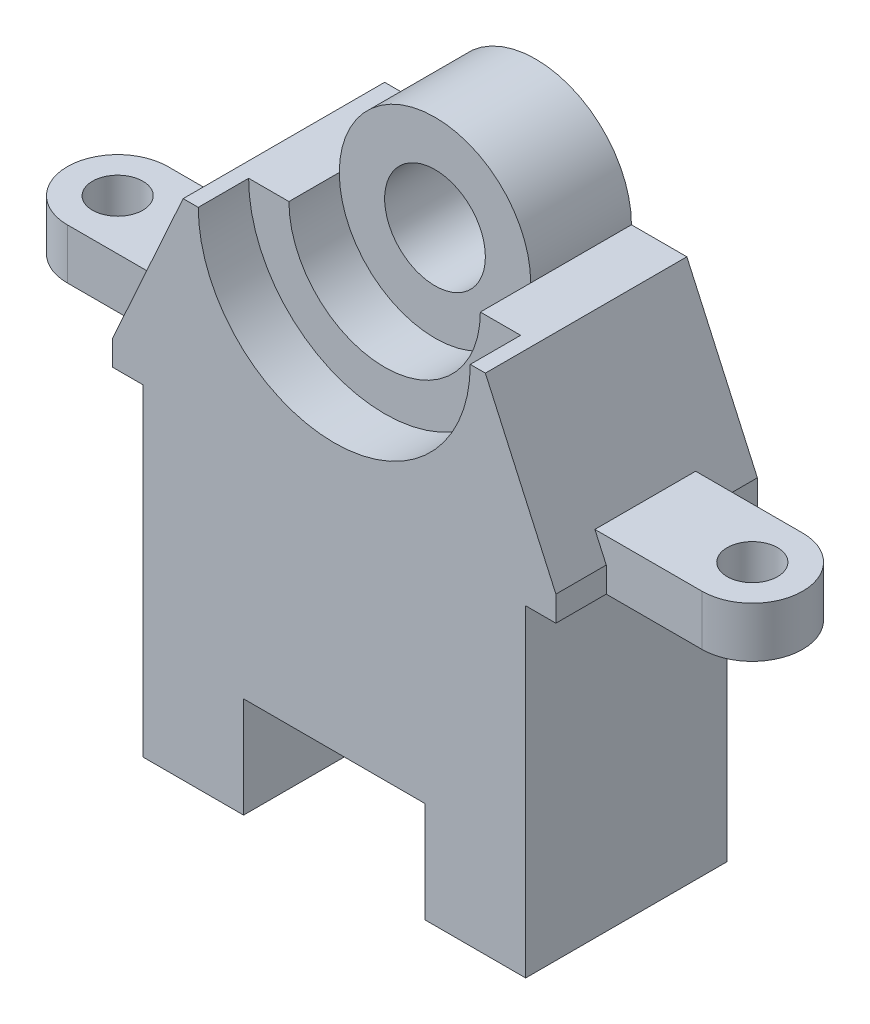
ISO-10303-21;
HEADER;
FILE_DESCRIPTION(('STEP AP214'),'2;1');
FILE_NAME('part.step','',(''),(''),'','','');
FILE_SCHEMA(('AUTOMOTIVE_DESIGN { 1 0 10303 214 1 1 1 1 }'));
ENDSEC;
DATA;
#1=APPLICATION_CONTEXT('core data for automotive mechanical design processes');
#2=APPLICATION_PROTOCOL_DEFINITION('international standard','automotive_design',2000,#1);
#3=PRODUCT_CONTEXT('',#1,'mechanical');
#4=PRODUCT('Part','Part','',(#3));
#5=PRODUCT_RELATED_PRODUCT_CATEGORY('part','',(#4));
#6=PRODUCT_DEFINITION_FORMATION('','',#4);
#7=PRODUCT_DEFINITION_CONTEXT('part definition',#1,'design');
#8=PRODUCT_DEFINITION('design','',#6,#7);
#9=PRODUCT_DEFINITION_SHAPE('','',#8);
#10=(LENGTH_UNIT() NAMED_UNIT(*) SI_UNIT(.MILLI.,.METRE.));
#11=(NAMED_UNIT(*) PLANE_ANGLE_UNIT() SI_UNIT($,.RADIAN.));
#12=(NAMED_UNIT(*) SI_UNIT($,.STERADIAN.) SOLID_ANGLE_UNIT());
#13=UNCERTAINTY_MEASURE_WITH_UNIT(LENGTH_MEASURE(1.E-05),#10,'distance_accuracy_value','');
#14=(GEOMETRIC_REPRESENTATION_CONTEXT(3) GLOBAL_UNCERTAINTY_ASSIGNED_CONTEXT((#13)) GLOBAL_UNIT_ASSIGNED_CONTEXT((#10,
#11,#12)) REPRESENTATION_CONTEXT('',''));
#15=CARTESIAN_POINT('',(0.,0.,0.));
#16=DIRECTION('',(0.,0.,1.));
#17=DIRECTION('',(1.,0.,0.));
#18=AXIS2_PLACEMENT_3D('',#15,#16,#17);
#19=CARTESIAN_POINT('',(44.,37.,20.));
#20=DIRECTION('',(-1.,0.,0.));
#21=DIRECTION('',(0.,0.,1.));
#22=AXIS2_PLACEMENT_3D('',#19,#20,#21);
#23=PLANE('',#22);
#24=DIRECTION('',(0.,1.,0.));
#25=VECTOR('',#24,1.);
#26=CARTESIAN_POINT('',(44.,37.,-10.));
#27=LINE('',#26,#25);
#28=CARTESIAN_POINT('',(44.,32.,-10.));
#29=VERTEX_POINT('',#28);
#30=CARTESIAN_POINT('',(44.,37.,-10.));
#31=VERTEX_POINT('',#30);
#32=EDGE_CURVE('E58',#29,#31,#27,.T.);
#33=ORIENTED_EDGE('',*,*,#32,.F.);
#34=DIRECTION('',(0.,0.,-1.));
#35=VECTOR('',#34,1.);
#36=CARTESIAN_POINT('',(44.,32.,20.));
#37=LINE('',#36,#35);
#38=CARTESIAN_POINT('',(44.,32.,-20.));
#39=VERTEX_POINT('',#38);
#40=EDGE_CURVE('E459',#29,#39,#37,.T.);
#41=ORIENTED_EDGE('',*,*,#40,.T.);
#42=DIRECTION('',(0.,1.,0.));
#43=VECTOR('',#42,1.);
#44=CARTESIAN_POINT('',(44.,37.,-20.));
#45=LINE('',#44,#43);
#46=CARTESIAN_POINT('',(44.,37.,-20.));
#47=VERTEX_POINT('',#46);
#48=EDGE_CURVE('E386',#39,#47,#45,.T.);
#49=ORIENTED_EDGE('',*,*,#48,.T.);
#50=DIRECTION('',(0.,0.,-1.));
#51=VECTOR('',#50,1.);
#52=CARTESIAN_POINT('',(44.,37.,20.));
#53=LINE('',#52,#51);
#54=EDGE_CURVE('E457',#31,#47,#53,.T.);
#55=ORIENTED_EDGE('',*,*,#54,.F.);
#56=EDGE_LOOP('',(#33,#41,#49,#55));
#57=FACE_BOUND('',#56,.T.);
#58=ADVANCED_FACE('F44',(#57),#23,.F.);
#59=DIRECTION('',(0.,-1.,0.));
#60=VECTOR('',#59,1.);
#61=CARTESIAN_POINT('',(44.,37.,10.));
#62=LINE('',#61,#60);
#63=CARTESIAN_POINT('',(44.,37.,10.));
#64=VERTEX_POINT('',#63);
#65=CARTESIAN_POINT('',(44.,32.,10.));
#66=VERTEX_POINT('',#65);
#67=EDGE_CURVE('E274',#64,#66,#62,.T.);
#68=ORIENTED_EDGE('',*,*,#67,.F.);
#69=CARTESIAN_POINT('',(44.,37.,20.));
#70=VERTEX_POINT('',#69);
#71=EDGE_CURVE('E460',#70,#64,#53,.T.);
#72=ORIENTED_EDGE('',*,*,#71,.F.);
#73=DIRECTION('',(0.,1.,0.));
#74=VECTOR('',#73,1.);
#75=CARTESIAN_POINT('',(44.,37.,20.));
#76=LINE('',#75,#74);
#77=CARTESIAN_POINT('',(44.,32.,20.));
#78=VERTEX_POINT('',#77);
#79=EDGE_CURVE('E357',#78,#70,#76,.T.);
#80=ORIENTED_EDGE('',*,*,#79,.F.);
#81=EDGE_CURVE('E69',#78,#66,#37,.T.);
#82=ORIENTED_EDGE('',*,*,#81,.T.);
#83=EDGE_LOOP('',(#68,#72,#80,#82));
#84=FACE_BOUND('',#83,.T.);
#85=ADVANCED_FACE('F476',(#84),#23,.F.);
#86=CARTESIAN_POINT('',(30.,68.,20.));
#87=DIRECTION('',(-0.911370599658675,-0.411586722426498,0.));
#88=DIRECTION('',(0.411586722426498,-0.911370599658675,0.));
#89=AXIS2_PLACEMENT_3D('',#86,#87,#88);
#90=PLANE('',#89);
#91=DIRECTION('',(-0.411586722426498,0.911370599658675,0.));
#92=VECTOR('',#91,1.);
#93=CARTESIAN_POINT('',(30.,68.,-10.));
#94=LINE('',#93,#92);
#95=CARTESIAN_POINT('',(41.741935483871,42.,-10.));
#96=VERTEX_POINT('',#95);
#97=EDGE_CURVE('E11',#31,#96,#94,.T.);
#98=ORIENTED_EDGE('',*,*,#97,.F.);
#99=ORIENTED_EDGE('',*,*,#54,.T.);
#100=DIRECTION('',(-0.411586722426498,0.911370599658675,0.));
#101=VECTOR('',#100,1.);
#102=CARTESIAN_POINT('',(30.,68.,-20.));
#103=LINE('',#102,#101);
#104=CARTESIAN_POINT('',(30.,68.,-20.));
#105=VERTEX_POINT('',#104);
#106=EDGE_CURVE('E394',#47,#105,#103,.T.);
#107=ORIENTED_EDGE('',*,*,#106,.T.);
#108=DIRECTION('',(0.,0.,-1.));
#109=VECTOR('',#108,1.);
#110=CARTESIAN_POINT('',(30.,68.,20.));
#111=LINE('',#110,#109);
#112=CARTESIAN_POINT('',(30.,68.,20.));
#113=VERTEX_POINT('',#112);
#114=EDGE_CURVE('E454',#113,#105,#111,.T.);
#115=ORIENTED_EDGE('',*,*,#114,.F.);
#116=DIRECTION('',(-0.411586722426498,0.911370599658675,0.));
#117=VECTOR('',#116,1.);
#118=CARTESIAN_POINT('',(30.,68.,20.));
#119=LINE('',#118,#117);
#120=EDGE_CURVE('E360',#70,#113,#119,.T.);
#121=ORIENTED_EDGE('',*,*,#120,.F.);
#122=ORIENTED_EDGE('',*,*,#71,.T.);
#123=DIRECTION('',(0.411586722426498,-0.911370599658675,0.));
#124=VECTOR('',#123,1.);
#125=CARTESIAN_POINT('',(30.,68.,10.));
#126=LINE('',#125,#124);
#127=CARTESIAN_POINT('',(41.741935483871,42.,10.));
#128=VERTEX_POINT('',#127);
#129=EDGE_CURVE('E472',#128,#64,#126,.T.);
#130=ORIENTED_EDGE('',*,*,#129,.F.);
#131=DIRECTION('',(0.,0.,1.));
#132=VECTOR('',#131,1.);
#133=CARTESIAN_POINT('',(41.741935483871,42.,20.));
#134=LINE('',#133,#132);
#135=EDGE_CURVE('E52',#96,#128,#134,.T.);
#136=ORIENTED_EDGE('',*,*,#135,.F.);
#137=EDGE_LOOP('',(#98,#99,#107,#115,#121,#122,#130,#136));
#138=FACE_BOUND('',#137,.T.);
#139=ADVANCED_FACE('F475',(#138),#90,.F.);
#140=CARTESIAN_POINT('',(-44.,32.,20.));
#141=DIRECTION('',(1.,0.,0.));
#142=DIRECTION('',(0.,0.,-1.));
#143=AXIS2_PLACEMENT_3D('',#140,#141,#142);
#144=PLANE('',#143);
#145=DIRECTION('',(0.,0.,-1.));
#146=VECTOR('',#145,1.);
#147=CARTESIAN_POINT('',(-44.,37.,20.));
#148=LINE('',#147,#146);
#149=CARTESIAN_POINT('',(-44.,37.,20.));
#150=VERTEX_POINT('',#149);
#151=CARTESIAN_POINT('',(-44.,37.,10.));
#152=VERTEX_POINT('',#151);
#153=EDGE_CURVE('E449',#150,#152,#148,.T.);
#154=ORIENTED_EDGE('',*,*,#153,.T.);
#155=DIRECTION('',(0.,-1.,0.));
#156=VECTOR('',#155,1.);
#157=CARTESIAN_POINT('',(-44.,32.,10.));
#158=LINE('',#157,#156);
#159=CARTESIAN_POINT('',(-44.,32.,10.));
#160=VERTEX_POINT('',#159);
#161=EDGE_CURVE('E315',#152,#160,#158,.T.);
#162=ORIENTED_EDGE('',*,*,#161,.T.);
#163=DIRECTION('',(0.,0.,-1.));
#164=VECTOR('',#163,1.);
#165=CARTESIAN_POINT('',(-44.,32.,20.));
#166=LINE('',#165,#164);
#167=CARTESIAN_POINT('',(-44.,32.,20.));
#168=VERTEX_POINT('',#167);
#169=EDGE_CURVE('E444',#168,#160,#166,.T.);
#170=ORIENTED_EDGE('',*,*,#169,.F.);
#171=DIRECTION('',(0.,-1.,0.));
#172=VECTOR('',#171,1.);
#173=CARTESIAN_POINT('',(-44.,32.,20.));
#174=LINE('',#173,#172);
#175=EDGE_CURVE('E366',#150,#168,#174,.T.);
#176=ORIENTED_EDGE('',*,*,#175,.F.);
#177=EDGE_LOOP('',(#154,#162,#170,#176));
#178=FACE_BOUND('',#177,.T.);
#179=ADVANCED_FACE('F482',(#178),#144,.F.);
#180=CARTESIAN_POINT('',(-30.,68.,20.));
#181=DIRECTION('',(0.,-1.,0.));
#182=DIRECTION('',(0.,0.,-1.));
#183=AXIS2_PLACEMENT_3D('',#180,#181,#182);
#184=PLANE('',#183);
#185=DIRECTION('',(-1.,0.,0.));
#186=VECTOR('',#185,1.);
#187=CARTESIAN_POINT('',(-30.,68.,-20.));
#188=LINE('',#187,#186);
#189=CARTESIAN_POINT('',(19.,68.,-20.));
#190=VERTEX_POINT('',#189);
#191=EDGE_CURVE('E391',#105,#190,#188,.T.);
#192=ORIENTED_EDGE('',*,*,#191,.T.);
#193=DIRECTION('',(0.,0.,1.));
#194=VECTOR('',#193,1.);
#195=CARTESIAN_POINT('',(19.,68.,-73.7401153701776));
#196=LINE('',#195,#194);
#197=CARTESIAN_POINT('',(19.,68.,0.));
#198=VERTEX_POINT('',#197);
#199=EDGE_CURVE('E335',#190,#198,#196,.T.);
#200=ORIENTED_EDGE('',*,*,#199,.T.);
#201=DIRECTION('',(0.,0.,1.));
#202=VECTOR('',#201,1.);
#203=CARTESIAN_POINT('',(19.,68.,0.));
#204=LINE('',#203,#202);
#205=CARTESIAN_POINT('',(19.,68.,10.));
#206=VERTEX_POINT('',#205);
#207=EDGE_CURVE('E341',#198,#206,#204,.T.);
#208=ORIENTED_EDGE('',*,*,#207,.T.);
#209=DIRECTION('',(-1.,0.,0.));
#210=VECTOR('',#209,1.);
#211=CARTESIAN_POINT('',(-30.,68.,10.));
#212=LINE('',#211,#210);
#213=CARTESIAN_POINT('',(27.,68.,10.));
#214=VERTEX_POINT('',#213);
#215=EDGE_CURVE('E461',#214,#206,#212,.T.);
#216=ORIENTED_EDGE('',*,*,#215,.F.);
#217=DIRECTION('',(0.,0.,1.));
#218=VECTOR('',#217,1.);
#219=CARTESIAN_POINT('',(27.,68.,10.));
#220=LINE('',#219,#218);
#221=CARTESIAN_POINT('',(27.,68.,20.));
#222=VERTEX_POINT('',#221);
#223=EDGE_CURVE('E348',#214,#222,#220,.T.);
#224=ORIENTED_EDGE('',*,*,#223,.T.);
#225=DIRECTION('',(-1.,0.,0.));
#226=VECTOR('',#225,1.);
#227=CARTESIAN_POINT('',(-30.,68.,20.));
#228=LINE('',#227,#226);
#229=EDGE_CURVE('E361',#113,#222,#228,.T.);
#230=ORIENTED_EDGE('',*,*,#229,.F.);
#231=ORIENTED_EDGE('',*,*,#114,.T.);
#232=EDGE_LOOP('',(#192,#200,#208,#216,#224,#230,#231));
#233=FACE_BOUND('',#232,.T.);
#234=ADVANCED_FACE('F495',(#233),#184,.F.);
#235=CARTESIAN_POINT('',(44.,32.,20.));
#236=DIRECTION('',(0.,1.,0.));
#237=DIRECTION('',(0.,0.,1.));
#238=AXIS2_PLACEMENT_3D('',#235,#236,#237);
#239=PLANE('',#238);
#240=DIRECTION('',(0.,0.,-1.));
#241=VECTOR('',#240,1.);
#242=CARTESIAN_POINT('',(38.,32.,20.));
#243=LINE('',#242,#241);
#244=CARTESIAN_POINT('',(38.,32.,20.));
#245=VERTEX_POINT('',#244);
#246=CARTESIAN_POINT('',(38.,32.,-20.));
#247=VERTEX_POINT('',#246);
#248=EDGE_CURVE('E387',#245,#247,#243,.T.);
#249=ORIENTED_EDGE('',*,*,#248,.T.);
#250=DIRECTION('',(1.,0.,0.));
#251=VECTOR('',#250,1.);
#252=CARTESIAN_POINT('',(44.,32.,-20.));
#253=LINE('',#252,#251);
#254=EDGE_CURVE('E352',#247,#39,#253,.T.);
#255=ORIENTED_EDGE('',*,*,#254,.T.);
#256=ORIENTED_EDGE('',*,*,#40,.F.);
#257=DIRECTION('',(-1.,0.,0.));
#258=VECTOR('',#257,1.);
#259=CARTESIAN_POINT('',(63.,32.,-10.));
#260=LINE('',#259,#258);
#261=CARTESIAN_POINT('',(63.,32.,-10.));
#262=VERTEX_POINT('',#261);
#263=EDGE_CURVE('E265',#262,#29,#260,.T.);
#264=ORIENTED_EDGE('',*,*,#263,.F.);
#265=CARTESIAN_POINT('',(63.,32.,0.));
#266=DIRECTION('',(0.,1.,0.));
#267=DIRECTION('',(0.,0.,-1.));
#268=AXIS2_PLACEMENT_3D('',#265,#266,#267);
#269=CIRCLE('',#268,10.);
#270=CARTESIAN_POINT('',(63.,32.,10.));
#271=VERTEX_POINT('',#270);
#272=EDGE_CURVE('E271',#271,#262,#269,.T.);
#273=ORIENTED_EDGE('',*,*,#272,.F.);
#274=DIRECTION('',(1.,0.,0.));
#275=VECTOR('',#274,1.);
#276=CARTESIAN_POINT('',(44.,32.,10.));
#277=LINE('',#276,#275);
#278=EDGE_CURVE('E255',#66,#271,#277,.T.);
#279=ORIENTED_EDGE('',*,*,#278,.F.);
#280=ORIENTED_EDGE('',*,*,#81,.F.);
#281=DIRECTION('',(1.,0.,0.));
#282=VECTOR('',#281,1.);
#283=CARTESIAN_POINT('',(44.,32.,20.));
#284=LINE('',#283,#282);
#285=EDGE_CURVE('E355',#245,#78,#284,.T.);
#286=ORIENTED_EDGE('',*,*,#285,.F.);
#287=EDGE_LOOP('',(#249,#255,#256,#264,#273,#279,#280,#286));
#288=FACE_BOUND('',#287,.T.);
#289=CARTESIAN_POINT('',(63.,32.,0.));
#290=DIRECTION('',(0.,1.,0.));
#291=DIRECTION('',(0.,0.,-1.));
#292=AXIS2_PLACEMENT_3D('',#289,#290,#291);
#293=CIRCLE('',#292,5.);
#294=CARTESIAN_POINT('',(63.,32.,-5.));
#295=VERTEX_POINT('',#294);
#296=EDGE_CURVE('E270',#295,#295,#293,.T.);
#297=ORIENTED_EDGE('',*,*,#296,.T.);
#298=EDGE_LOOP('',(#297));
#299=FACE_BOUND('',#298,.T.);
#300=ADVANCED_FACE('F50',(#288,#299),#239,.F.);
#301=DIRECTION('',(0.,0.,1.));
#302=VECTOR('',#301,1.);
#303=CARTESIAN_POINT('',(-19.,68.,0.));
#304=LINE('',#303,#302);
#305=CARTESIAN_POINT('',(-19.,68.,10.));
#306=VERTEX_POINT('',#305);
#307=CARTESIAN_POINT('',(-19.,68.,0.));
#308=VERTEX_POINT('',#307);
#309=EDGE_CURVE('E337',#306,#308,#304,.F.);
#310=ORIENTED_EDGE('',*,*,#309,.T.);
#311=DIRECTION('',(0.,0.,1.));
#312=VECTOR('',#311,1.);
#313=CARTESIAN_POINT('',(-19.,68.,-73.7401153701776));
#314=LINE('',#313,#312);
#315=CARTESIAN_POINT('',(-19.,68.,-20.));
#316=VERTEX_POINT('',#315);
#317=EDGE_CURVE('E328',#308,#316,#314,.F.);
#318=ORIENTED_EDGE('',*,*,#317,.T.);
#319=CARTESIAN_POINT('',(-30.,68.,-20.));
#320=VERTEX_POINT('',#319);
#321=EDGE_CURVE('E395',#316,#320,#188,.T.);
#322=ORIENTED_EDGE('',*,*,#321,.T.);
#323=DIRECTION('',(0.,0.,-1.));
#324=VECTOR('',#323,1.);
#325=CARTESIAN_POINT('',(-30.,68.,20.));
#326=LINE('',#325,#324);
#327=CARTESIAN_POINT('',(-30.,68.,20.));
#328=VERTEX_POINT('',#327);
#329=EDGE_CURVE('E446',#328,#320,#326,.T.);
#330=ORIENTED_EDGE('',*,*,#329,.F.);
#331=CARTESIAN_POINT('',(-27.,68.,20.));
#332=VERTEX_POINT('',#331);
#333=EDGE_CURVE('E362',#332,#328,#228,.T.);
#334=ORIENTED_EDGE('',*,*,#333,.F.);
#335=DIRECTION('',(0.,0.,1.));
#336=VECTOR('',#335,1.);
#337=CARTESIAN_POINT('',(-27.,68.,10.));
#338=LINE('',#337,#336);
#339=CARTESIAN_POINT('',(-27.,68.,10.));
#340=VERTEX_POINT('',#339);
#341=EDGE_CURVE('E350',#332,#340,#338,.F.);
#342=ORIENTED_EDGE('',*,*,#341,.T.);
#343=EDGE_CURVE('E465',#306,#340,#212,.T.);
#344=ORIENTED_EDGE('',*,*,#343,.F.);
#345=EDGE_LOOP('',(#310,#318,#322,#330,#334,#342,#344));
#346=FACE_BOUND('',#345,.T.);
#347=ADVANCED_FACE('F490',(#346),#184,.F.);
#348=CARTESIAN_POINT('',(-44.,37.,20.));
#349=DIRECTION('',(0.911370599658675,-0.411586722426498,0.));
#350=DIRECTION('',(0.411586722426498,0.911370599658675,0.));
#351=AXIS2_PLACEMENT_3D('',#348,#349,#350);
#352=PLANE('',#351);
#353=DIRECTION('',(0.,0.,-1.));
#354=VECTOR('',#353,1.);
#355=CARTESIAN_POINT('',(-41.741935483871,42.,20.));
#356=LINE('',#355,#354);
#357=CARTESIAN_POINT('',(-41.741935483871,42.,10.));
#358=VERTEX_POINT('',#357);
#359=CARTESIAN_POINT('',(-41.741935483871,42.,-10.));
#360=VERTEX_POINT('',#359);
#361=EDGE_CURVE('E470',#358,#360,#356,.T.);
#362=ORIENTED_EDGE('',*,*,#361,.F.);
#363=DIRECTION('',(-0.411586722426498,-0.911370599658675,0.));
#364=VECTOR('',#363,1.);
#365=CARTESIAN_POINT('',(-44.,37.,10.));
#366=LINE('',#365,#364);
#367=EDGE_CURVE('E312',#358,#152,#366,.T.);
#368=ORIENTED_EDGE('',*,*,#367,.T.);
#369=ORIENTED_EDGE('',*,*,#153,.F.);
#370=DIRECTION('',(-0.411586722426498,-0.911370599658675,0.));
#371=VECTOR('',#370,1.);
#372=CARTESIAN_POINT('',(-44.,37.,20.));
#373=LINE('',#372,#371);
#374=EDGE_CURVE('E368',#328,#150,#373,.T.);
#375=ORIENTED_EDGE('',*,*,#374,.F.);
#376=ORIENTED_EDGE('',*,*,#329,.T.);
#377=DIRECTION('',(-0.411586722426498,-0.911370599658675,0.));
#378=VECTOR('',#377,1.);
#379=CARTESIAN_POINT('',(-44.,37.,-20.));
#380=LINE('',#379,#378);
#381=CARTESIAN_POINT('',(-44.,37.,-20.));
#382=VERTEX_POINT('',#381);
#383=EDGE_CURVE('E399',#320,#382,#380,.T.);
#384=ORIENTED_EDGE('',*,*,#383,.T.);
#385=CARTESIAN_POINT('',(-44.,37.,-10.));
#386=VERTEX_POINT('',#385);
#387=EDGE_CURVE('E448',#386,#382,#148,.T.);
#388=ORIENTED_EDGE('',*,*,#387,.F.);
#389=DIRECTION('',(0.411586722426498,0.911370599658675,0.));
#390=VECTOR('',#389,1.);
#391=CARTESIAN_POINT('',(-44.,37.,-10.));
#392=LINE('',#391,#390);
#393=EDGE_CURVE('E310',#386,#360,#392,.T.);
#394=ORIENTED_EDGE('',*,*,#393,.T.);
#395=EDGE_LOOP('',(#362,#368,#369,#375,#376,#384,#388,#394));
#396=FACE_BOUND('',#395,.T.);
#397=ADVANCED_FACE('F489',(#396),#352,.F.);
#398=CARTESIAN_POINT('',(-44.,32.,-10.));
#399=VERTEX_POINT('',#398);
#400=CARTESIAN_POINT('',(-44.,32.,-20.));
#401=VERTEX_POINT('',#400);
#402=EDGE_CURVE('E445',#399,#401,#166,.T.);
#403=ORIENTED_EDGE('',*,*,#402,.F.);
#404=DIRECTION('',(0.,1.,0.));
#405=VECTOR('',#404,1.);
#406=CARTESIAN_POINT('',(-44.,32.,-10.));
#407=LINE('',#406,#405);
#408=EDGE_CURVE('E303',#399,#386,#407,.T.);
#409=ORIENTED_EDGE('',*,*,#408,.T.);
#410=ORIENTED_EDGE('',*,*,#387,.T.);
#411=DIRECTION('',(0.,-1.,0.));
#412=VECTOR('',#411,1.);
#413=CARTESIAN_POINT('',(-44.,32.,-20.));
#414=LINE('',#413,#412);
#415=EDGE_CURVE('E402',#382,#401,#414,.T.);
#416=ORIENTED_EDGE('',*,*,#415,.T.);
#417=EDGE_LOOP('',(#403,#409,#410,#416));
#418=FACE_BOUND('',#417,.T.);
#419=ADVANCED_FACE('F494',(#418),#144,.F.);
#420=CARTESIAN_POINT('',(-38.,32.,20.));
#421=DIRECTION('',(0.,1.,0.));
#422=DIRECTION('',(0.,0.,1.));
#423=AXIS2_PLACEMENT_3D('',#420,#421,#422);
#424=PLANE('',#423);
#425=DIRECTION('',(1.,0.,0.));
#426=VECTOR('',#425,1.);
#427=CARTESIAN_POINT('',(-38.,32.,-20.));
#428=LINE('',#427,#426);
#429=CARTESIAN_POINT('',(-38.,32.,-20.));
#430=VERTEX_POINT('',#429);
#431=EDGE_CURVE('E404',#401,#430,#428,.T.);
#432=ORIENTED_EDGE('',*,*,#431,.T.);
#433=DIRECTION('',(0.,0.,-1.));
#434=VECTOR('',#433,1.);
#435=CARTESIAN_POINT('',(-38.,32.,20.));
#436=LINE('',#435,#434);
#437=CARTESIAN_POINT('',(-38.,32.,20.));
#438=VERTEX_POINT('',#437);
#439=EDGE_CURVE('E439',#438,#430,#436,.T.);
#440=ORIENTED_EDGE('',*,*,#439,.F.);
#441=DIRECTION('',(1.,0.,0.));
#442=VECTOR('',#441,1.);
#443=CARTESIAN_POINT('',(-38.,32.,20.));
#444=LINE('',#443,#442);
#445=EDGE_CURVE('E367',#168,#438,#444,.T.);
#446=ORIENTED_EDGE('',*,*,#445,.F.);
#447=ORIENTED_EDGE('',*,*,#169,.T.);
#448=DIRECTION('',(-1.,0.,0.));
#449=VECTOR('',#448,1.);
#450=CARTESIAN_POINT('',(-63.,32.,10.));
#451=LINE('',#450,#449);
#452=CARTESIAN_POINT('',(-63.,32.,10.));
#453=VERTEX_POINT('',#452);
#454=EDGE_CURVE('E290',#160,#453,#451,.T.);
#455=ORIENTED_EDGE('',*,*,#454,.T.);
#456=CARTESIAN_POINT('',(-63.,32.,0.));
#457=DIRECTION('',(0.,-1.,0.));
#458=DIRECTION('',(0.,0.,-1.));
#459=AXIS2_PLACEMENT_3D('',#456,#457,#458);
#460=CIRCLE('',#459,10.);
#461=CARTESIAN_POINT('',(-63.,32.,-10.));
#462=VERTEX_POINT('',#461);
#463=EDGE_CURVE('E282',#453,#462,#460,.T.);
#464=ORIENTED_EDGE('',*,*,#463,.T.);
#465=DIRECTION('',(1.,0.,0.));
#466=VECTOR('',#465,1.);
#467=CARTESIAN_POINT('',(-38.,32.,-10.));
#468=LINE('',#467,#466);
#469=EDGE_CURVE('E297',#462,#399,#468,.T.);
#470=ORIENTED_EDGE('',*,*,#469,.T.);
#471=ORIENTED_EDGE('',*,*,#402,.T.);
#472=EDGE_LOOP('',(#432,#440,#446,#447,#455,#464,#470,#471));
#473=FACE_BOUND('',#472,.T.);
#474=CARTESIAN_POINT('',(-63.,32.,0.));
#475=DIRECTION('',(0.,-1.,0.));
#476=DIRECTION('',(0.,0.,-1.));
#477=AXIS2_PLACEMENT_3D('',#474,#475,#476);
#478=CIRCLE('',#477,5.);
#479=CARTESIAN_POINT('',(-63.,32.,-5.));
#480=VERTEX_POINT('',#479);
#481=EDGE_CURVE('E276',#480,#480,#478,.T.);
#482=ORIENTED_EDGE('',*,*,#481,.F.);
#483=EDGE_LOOP('',(#482));
#484=FACE_BOUND('',#483,.T.);
#485=ADVANCED_FACE('F496',(#473,#484),#424,.F.);
#486=CARTESIAN_POINT('',(-38.,-32.,20.));
#487=DIRECTION('',(1.,0.,0.));
#488=DIRECTION('',(0.,0.,-1.));
#489=AXIS2_PLACEMENT_3D('',#486,#487,#488);
#490=PLANE('',#489);
#491=DIRECTION('',(0.,-1.,0.));
#492=VECTOR('',#491,1.);
#493=CARTESIAN_POINT('',(-38.,-32.,-20.));
#494=LINE('',#493,#492);
#495=CARTESIAN_POINT('',(-38.,-32.,-20.));
#496=VERTEX_POINT('',#495);
#497=EDGE_CURVE('E409',#430,#496,#494,.T.);
#498=ORIENTED_EDGE('',*,*,#497,.T.);
#499=DIRECTION('',(0.,0.,-1.));
#500=VECTOR('',#499,1.);
#501=CARTESIAN_POINT('',(-38.,-32.,20.));
#502=LINE('',#501,#500);
#503=CARTESIAN_POINT('',(-38.,-32.,20.));
#504=VERTEX_POINT('',#503);
#505=EDGE_CURVE('E440',#504,#496,#502,.T.);
#506=ORIENTED_EDGE('',*,*,#505,.F.);
#507=DIRECTION('',(0.,-1.,0.));
#508=VECTOR('',#507,1.);
#509=CARTESIAN_POINT('',(-38.,-32.,20.));
#510=LINE('',#509,#508);
#511=EDGE_CURVE('E375',#438,#504,#510,.T.);
#512=ORIENTED_EDGE('',*,*,#511,.F.);
#513=ORIENTED_EDGE('',*,*,#439,.T.);
#514=EDGE_LOOP('',(#498,#506,#512,#513));
#515=FACE_BOUND('',#514,.T.);
#516=ADVANCED_FACE('F502',(#515),#490,.F.);
#517=CARTESIAN_POINT('',(-38.,-32.,20.));
#518=DIRECTION('',(0.,1.,0.));
#519=DIRECTION('',(0.,0.,1.));
#520=AXIS2_PLACEMENT_3D('',#517,#518,#519);
#521=PLANE('',#520);
#522=DIRECTION('',(1.,0.,0.));
#523=VECTOR('',#522,1.);
#524=CARTESIAN_POINT('',(-38.,-32.,-20.));
#525=LINE('',#524,#523);
#526=CARTESIAN_POINT('',(-18.,-32.,-20.));
#527=VERTEX_POINT('',#526);
#528=EDGE_CURVE('E410',#496,#527,#525,.T.);
#529=ORIENTED_EDGE('',*,*,#528,.T.);
#530=DIRECTION('',(0.,0.,-1.));
#531=VECTOR('',#530,1.);
#532=CARTESIAN_POINT('',(-18.,-32.,20.));
#533=LINE('',#532,#531);
#534=CARTESIAN_POINT('',(-18.,-32.,20.));
#535=VERTEX_POINT('',#534);
#536=EDGE_CURVE('E432',#535,#527,#533,.T.);
#537=ORIENTED_EDGE('',*,*,#536,.F.);
#538=DIRECTION('',(1.,0.,0.));
#539=VECTOR('',#538,1.);
#540=CARTESIAN_POINT('',(-38.,-32.,20.));
#541=LINE('',#540,#539);
#542=EDGE_CURVE('E372',#504,#535,#541,.T.);
#543=ORIENTED_EDGE('',*,*,#542,.F.);
#544=ORIENTED_EDGE('',*,*,#505,.T.);
#545=EDGE_LOOP('',(#529,#537,#543,#544));
#546=FACE_BOUND('',#545,.T.);
#547=ADVANCED_FACE('F507',(#546),#521,.F.);
#548=CARTESIAN_POINT('',(-18.,-32.,20.));
#549=DIRECTION('',(-1.,0.,0.));
#550=DIRECTION('',(0.,0.,1.));
#551=AXIS2_PLACEMENT_3D('',#548,#549,#550);
#552=PLANE('',#551);
#553=DIRECTION('',(0.,1.,0.));
#554=VECTOR('',#553,1.);
#555=CARTESIAN_POINT('',(-18.,-32.,-20.));
#556=LINE('',#555,#554);
#557=CARTESIAN_POINT('',(-18.,-12.,-20.));
#558=VERTEX_POINT('',#557);
#559=EDGE_CURVE('E411',#527,#558,#556,.T.);
#560=ORIENTED_EDGE('',*,*,#559,.T.);
#561=DIRECTION('',(0.,0.,-1.));
#562=VECTOR('',#561,1.);
#563=CARTESIAN_POINT('',(-18.,-12.,20.));
#564=LINE('',#563,#562);
#565=CARTESIAN_POINT('',(-18.,-12.,20.));
#566=VERTEX_POINT('',#565);
#567=EDGE_CURVE('E431',#566,#558,#564,.T.);
#568=ORIENTED_EDGE('',*,*,#567,.F.);
#569=DIRECTION('',(0.,1.,0.));
#570=VECTOR('',#569,1.);
#571=CARTESIAN_POINT('',(-18.,-32.,20.));
#572=LINE('',#571,#570);
#573=EDGE_CURVE('E376',#535,#566,#572,.T.);
#574=ORIENTED_EDGE('',*,*,#573,.F.);
#575=ORIENTED_EDGE('',*,*,#536,.T.);
#576=EDGE_LOOP('',(#560,#568,#574,#575));
#577=FACE_BOUND('',#576,.T.);
#578=ADVANCED_FACE('F512',(#577),#552,.F.);
#579=CARTESIAN_POINT('',(-18.,-12.,20.));
#580=DIRECTION('',(0.,1.,0.));
#581=DIRECTION('',(0.,0.,1.));
#582=AXIS2_PLACEMENT_3D('',#579,#580,#581);
#583=PLANE('',#582);
#584=DIRECTION('',(1.,0.,0.));
#585=VECTOR('',#584,1.);
#586=CARTESIAN_POINT('',(-18.,-12.,-20.));
#587=LINE('',#586,#585);
#588=CARTESIAN_POINT('',(18.,-12.,-20.));
#589=VERTEX_POINT('',#588);
#590=EDGE_CURVE('E414',#558,#589,#587,.T.);
#591=ORIENTED_EDGE('',*,*,#590,.T.);
#592=DIRECTION('',(0.,0.,-1.));
#593=VECTOR('',#592,1.);
#594=CARTESIAN_POINT('',(18.,-12.,20.));
#595=LINE('',#594,#593);
#596=CARTESIAN_POINT('',(18.,-12.,20.));
#597=VERTEX_POINT('',#596);
#598=EDGE_CURVE('E428',#597,#589,#595,.T.);
#599=ORIENTED_EDGE('',*,*,#598,.F.);
#600=DIRECTION('',(1.,0.,0.));
#601=VECTOR('',#600,1.);
#602=CARTESIAN_POINT('',(-18.,-12.,20.));
#603=LINE('',#602,#601);
#604=EDGE_CURVE('E378',#566,#597,#603,.T.);
#605=ORIENTED_EDGE('',*,*,#604,.F.);
#606=ORIENTED_EDGE('',*,*,#567,.T.);
#607=EDGE_LOOP('',(#591,#599,#605,#606));
#608=FACE_BOUND('',#607,.T.);
#609=ADVANCED_FACE('F513',(#608),#583,.F.);
#610=CARTESIAN_POINT('',(18.,-32.,20.));
#611=DIRECTION('',(1.,0.,0.));
#612=DIRECTION('',(0.,0.,-1.));
#613=AXIS2_PLACEMENT_3D('',#610,#611,#612);
#614=PLANE('',#613);
#615=DIRECTION('',(0.,-1.,0.));
#616=VECTOR('',#615,1.);
#617=CARTESIAN_POINT('',(18.,-32.,-20.));
#618=LINE('',#617,#616);
#619=CARTESIAN_POINT('',(18.,-32.,-20.));
#620=VERTEX_POINT('',#619);
#621=EDGE_CURVE('E415',#589,#620,#618,.T.);
#622=ORIENTED_EDGE('',*,*,#621,.T.);
#623=DIRECTION('',(0.,0.,-1.));
#624=VECTOR('',#623,1.);
#625=CARTESIAN_POINT('',(18.,-32.,20.));
#626=LINE('',#625,#624);
#627=CARTESIAN_POINT('',(18.,-32.,20.));
#628=VERTEX_POINT('',#627);
#629=EDGE_CURVE('E422',#628,#620,#626,.T.);
#630=ORIENTED_EDGE('',*,*,#629,.F.);
#631=DIRECTION('',(0.,-1.,0.));
#632=VECTOR('',#631,1.);
#633=CARTESIAN_POINT('',(18.,-32.,20.));
#634=LINE('',#633,#632);
#635=EDGE_CURVE('E379',#597,#628,#634,.T.);
#636=ORIENTED_EDGE('',*,*,#635,.F.);
#637=ORIENTED_EDGE('',*,*,#598,.T.);
#638=EDGE_LOOP('',(#622,#630,#636,#637));
#639=FACE_BOUND('',#638,.T.);
#640=ADVANCED_FACE('F520',(#639),#614,.F.);
#641=CARTESIAN_POINT('',(18.,-32.,20.));
#642=DIRECTION('',(0.,1.,0.));
#643=DIRECTION('',(0.,0.,1.));
#644=AXIS2_PLACEMENT_3D('',#641,#642,#643);
#645=PLANE('',#644);
#646=DIRECTION('',(1.,0.,0.));
#647=VECTOR('',#646,1.);
#648=CARTESIAN_POINT('',(18.,-32.,-20.));
#649=LINE('',#648,#647);
#650=CARTESIAN_POINT('',(38.,-32.,-20.));
#651=VERTEX_POINT('',#650);
#652=EDGE_CURVE('E417',#620,#651,#649,.T.);
#653=ORIENTED_EDGE('',*,*,#652,.T.);
#654=DIRECTION('',(0.,0.,-1.));
#655=VECTOR('',#654,1.);
#656=CARTESIAN_POINT('',(38.,-32.,20.));
#657=LINE('',#656,#655);
#658=CARTESIAN_POINT('',(38.,-32.,20.));
#659=VERTEX_POINT('',#658);
#660=EDGE_CURVE('E425',#659,#651,#657,.T.);
#661=ORIENTED_EDGE('',*,*,#660,.F.);
#662=DIRECTION('',(1.,0.,0.));
#663=VECTOR('',#662,1.);
#664=CARTESIAN_POINT('',(18.,-32.,20.));
#665=LINE('',#664,#663);
#666=EDGE_CURVE('E385',#628,#659,#665,.T.);
#667=ORIENTED_EDGE('',*,*,#666,.F.);
#668=ORIENTED_EDGE('',*,*,#629,.T.);
#669=EDGE_LOOP('',(#653,#661,#667,#668));
#670=FACE_BOUND('',#669,.T.);
#671=ADVANCED_FACE('F524',(#670),#645,.F.);
#672=CARTESIAN_POINT('',(38.,-32.,20.));
#673=DIRECTION('',(-1.,0.,0.));
#674=DIRECTION('',(0.,0.,1.));
#675=AXIS2_PLACEMENT_3D('',#672,#673,#674);
#676=PLANE('',#675);
#677=DIRECTION('',(0.,1.,0.));
#678=VECTOR('',#677,1.);
#679=CARTESIAN_POINT('',(38.,-32.,-20.));
#680=LINE('',#679,#678);
#681=EDGE_CURVE('E359',#651,#247,#680,.T.);
#682=ORIENTED_EDGE('',*,*,#681,.T.);
#683=ORIENTED_EDGE('',*,*,#248,.F.);
#684=DIRECTION('',(0.,1.,0.));
#685=VECTOR('',#684,1.);
#686=CARTESIAN_POINT('',(38.,-32.,20.));
#687=LINE('',#686,#685);
#688=EDGE_CURVE('E383',#659,#245,#687,.T.);
#689=ORIENTED_EDGE('',*,*,#688,.F.);
#690=ORIENTED_EDGE('',*,*,#660,.T.);
#691=EDGE_LOOP('',(#682,#683,#689,#690));
#692=FACE_BOUND('',#691,.T.);
#693=ADVANCED_FACE('F527',(#692),#676,.F.);
#694=CARTESIAN_POINT('',(0.,0.,20.));
#695=DIRECTION('',(0.,0.,-1.));
#696=DIRECTION('',(-1.,0.,0.));
#697=AXIS2_PLACEMENT_3D('',#694,#695,#696);
#698=PLANE('',#697);
#699=ORIENTED_EDGE('',*,*,#229,.T.);
#700=CARTESIAN_POINT('',(0.,68.,20.));
#701=DIRECTION('',(0.,0.,-1.));
#702=DIRECTION('',(-1.,0.,0.));
#703=AXIS2_PLACEMENT_3D('',#700,#701,#702);
#704=CIRCLE('',#703,27.);
#705=EDGE_CURVE('E463',#222,#332,#704,.T.);
#706=ORIENTED_EDGE('',*,*,#705,.T.);
#707=ORIENTED_EDGE('',*,*,#333,.T.);
#708=ORIENTED_EDGE('',*,*,#374,.T.);
#709=ORIENTED_EDGE('',*,*,#175,.T.);
#710=ORIENTED_EDGE('',*,*,#445,.T.);
#711=ORIENTED_EDGE('',*,*,#511,.T.);
#712=ORIENTED_EDGE('',*,*,#542,.T.);
#713=ORIENTED_EDGE('',*,*,#573,.T.);
#714=ORIENTED_EDGE('',*,*,#604,.T.);
#715=ORIENTED_EDGE('',*,*,#635,.T.);
#716=ORIENTED_EDGE('',*,*,#666,.T.);
#717=ORIENTED_EDGE('',*,*,#688,.T.);
#718=ORIENTED_EDGE('',*,*,#285,.T.);
#719=ORIENTED_EDGE('',*,*,#79,.T.);
#720=ORIENTED_EDGE('',*,*,#120,.T.);
#721=EDGE_LOOP('',(#699,#706,#707,#708,#709,#710,#711,#712,#713,#714,#715,#716,#717,#718,#719,#720));
#722=FACE_BOUND('',#721,.T.);
#723=ADVANCED_FACE('F533',(#722),#698,.F.);
#724=CARTESIAN_POINT('',(0.,0.,-20.));
#725=DIRECTION('',(0.,0.,-1.));
#726=DIRECTION('',(-1.,0.,0.));
#727=AXIS2_PLACEMENT_3D('',#724,#725,#726);
#728=PLANE('',#727);
#729=CARTESIAN_POINT('',(0.,68.,-20.));
#730=DIRECTION('',(0.,0.,1.));
#731=DIRECTION('',(1.,0.,0.));
#732=AXIS2_PLACEMENT_3D('',#729,#730,#731);
#733=CIRCLE('',#732,10.);
#734=CARTESIAN_POINT('',(10.,68.,-20.));
#735=VERTEX_POINT('',#734);
#736=EDGE_CURVE('E317',#735,#735,#733,.T.);
#737=ORIENTED_EDGE('',*,*,#736,.T.);
#738=EDGE_LOOP('',(#737));
#739=FACE_BOUND('',#738,.T.);
#740=ORIENTED_EDGE('',*,*,#321,.F.);
#741=CARTESIAN_POINT('',(0.,68.,-20.));
#742=DIRECTION('',(0.,0.,-1.));
#743=DIRECTION('',(-1.,0.,0.));
#744=AXIS2_PLACEMENT_3D('',#741,#742,#743);
#745=CIRCLE('',#744,19.);
#746=EDGE_CURVE('E330',#190,#316,#745,.F.);
#747=ORIENTED_EDGE('',*,*,#746,.F.);
#748=ORIENTED_EDGE('',*,*,#191,.F.);
#749=ORIENTED_EDGE('',*,*,#106,.F.);
#750=ORIENTED_EDGE('',*,*,#48,.F.);
#751=ORIENTED_EDGE('',*,*,#254,.F.);
#752=ORIENTED_EDGE('',*,*,#681,.F.);
#753=ORIENTED_EDGE('',*,*,#652,.F.);
#754=ORIENTED_EDGE('',*,*,#621,.F.);
#755=ORIENTED_EDGE('',*,*,#590,.F.);
#756=ORIENTED_EDGE('',*,*,#559,.F.);
#757=ORIENTED_EDGE('',*,*,#528,.F.);
#758=ORIENTED_EDGE('',*,*,#497,.F.);
#759=ORIENTED_EDGE('',*,*,#431,.F.);
#760=ORIENTED_EDGE('',*,*,#415,.F.);
#761=ORIENTED_EDGE('',*,*,#383,.F.);
#762=EDGE_LOOP('',(#740,#747,#748,#749,#750,#751,#752,#753,#754,#755,#756,#757,#758,#759,#760,#761));
#763=FACE_BOUND('',#762,.T.);
#764=ADVANCED_FACE('F531',(#739,#763),#728,.T.);
#765=CARTESIAN_POINT('',(0.,68.,10.));
#766=DIRECTION('',(0.,0.,1.));
#767=DIRECTION('',(1.,0.,0.));
#768=AXIS2_PLACEMENT_3D('',#765,#766,#767);
#769=PLANE('',#768);
#770=CARTESIAN_POINT('',(0.,68.,10.));
#771=DIRECTION('',(0.,0.,1.));
#772=DIRECTION('',(1.,0.,0.));
#773=AXIS2_PLACEMENT_3D('',#770,#771,#772);
#774=CIRCLE('',#773,19.);
#775=EDGE_CURVE('E469',#306,#206,#774,.T.);
#776=ORIENTED_EDGE('',*,*,#775,.F.);
#777=ORIENTED_EDGE('',*,*,#343,.T.);
#778=CARTESIAN_POINT('',(0.,68.,10.));
#779=DIRECTION('',(0.,0.,1.));
#780=DIRECTION('',(1.,0.,0.));
#781=AXIS2_PLACEMENT_3D('',#778,#779,#780);
#782=CIRCLE('',#781,27.);
#783=EDGE_CURVE('E343',#340,#214,#782,.T.);
#784=ORIENTED_EDGE('',*,*,#783,.T.);
#785=ORIENTED_EDGE('',*,*,#215,.T.);
#786=EDGE_LOOP('',(#776,#777,#784,#785));
#787=FACE_BOUND('',#786,.T.);
#788=ADVANCED_FACE('F536',(#787),#769,.T.);
#789=CARTESIAN_POINT('',(0.,68.,10.));
#790=DIRECTION('',(0.,0.,1.));
#791=DIRECTION('',(1.,0.,0.));
#792=AXIS2_PLACEMENT_3D('',#789,#790,#791);
#793=CYLINDRICAL_SURFACE('',#792,27.);
#794=ORIENTED_EDGE('',*,*,#783,.F.);
#795=ORIENTED_EDGE('',*,*,#341,.F.);
#796=ORIENTED_EDGE('',*,*,#705,.F.);
#797=ORIENTED_EDGE('',*,*,#223,.F.);
#798=EDGE_LOOP('',(#794,#795,#796,#797));
#799=FACE_BOUND('',#798,.T.);
#800=ADVANCED_FACE('F541',(#799),#793,.F.);
#801=CARTESIAN_POINT('',(0.,68.,0.));
#802=DIRECTION('',(0.,0.,1.));
#803=DIRECTION('',(1.,0.,0.));
#804=AXIS2_PLACEMENT_3D('',#801,#802,#803);
#805=PLANE('',#804);
#806=CARTESIAN_POINT('',(0.,68.,0.));
#807=DIRECTION('',(0.,0.,1.));
#808=DIRECTION('',(1.,0.,0.));
#809=AXIS2_PLACEMENT_3D('',#806,#807,#808);
#810=CIRCLE('',#809,10.);
#811=CARTESIAN_POINT('',(10.,68.,0.));
#812=VERTEX_POINT('',#811);
#813=EDGE_CURVE('E318',#812,#812,#810,.T.);
#814=ORIENTED_EDGE('',*,*,#813,.F.);
#815=EDGE_LOOP('',(#814));
#816=FACE_BOUND('',#815,.T.);
#817=CARTESIAN_POINT('',(0.,68.,0.));
#818=DIRECTION('',(0.,0.,1.));
#819=DIRECTION('',(1.,0.,0.));
#820=AXIS2_PLACEMENT_3D('',#817,#818,#819);
#821=CIRCLE('',#820,19.);
#822=EDGE_CURVE('E333',#308,#198,#821,.T.);
#823=ORIENTED_EDGE('',*,*,#822,.T.);
#824=CARTESIAN_POINT('',(0.,68.,0.));
#825=DIRECTION('',(0.,0.,1.));
#826=DIRECTION('',(1.,0.,0.));
#827=AXIS2_PLACEMENT_3D('',#824,#825,#826);
#828=CIRCLE('',#827,19.);
#829=EDGE_CURVE('E325',#198,#308,#828,.T.);
#830=ORIENTED_EDGE('',*,*,#829,.T.);
#831=EDGE_LOOP('',(#823,#830));
#832=FACE_BOUND('',#831,.T.);
#833=ADVANCED_FACE('F542',(#816,#832),#805,.T.);
#834=CARTESIAN_POINT('',(0.,68.,0.));
#835=DIRECTION('',(0.,0.,1.));
#836=DIRECTION('',(1.,0.,0.));
#837=AXIS2_PLACEMENT_3D('',#834,#835,#836);
#838=CYLINDRICAL_SURFACE('',#837,19.);
#839=ORIENTED_EDGE('',*,*,#822,.F.);
#840=ORIENTED_EDGE('',*,*,#309,.F.);
#841=ORIENTED_EDGE('',*,*,#775,.T.);
#842=ORIENTED_EDGE('',*,*,#207,.F.);
#843=EDGE_LOOP('',(#839,#840,#841,#842));
#844=FACE_BOUND('',#843,.T.);
#845=ADVANCED_FACE('F548',(#844),#838,.F.);
#846=CARTESIAN_POINT('',(0.,68.,-73.7401153701776));
#847=DIRECTION('',(0.,0.,1.));
#848=DIRECTION('',(1.,0.,0.));
#849=AXIS2_PLACEMENT_3D('',#846,#847,#848);
#850=CYLINDRICAL_SURFACE('',#849,19.);
#851=ORIENTED_EDGE('',*,*,#199,.F.);
#852=ORIENTED_EDGE('',*,*,#746,.T.);
#853=ORIENTED_EDGE('',*,*,#317,.F.);
#854=ORIENTED_EDGE('',*,*,#829,.F.);
#855=EDGE_LOOP('',(#851,#852,#853,#854));
#856=FACE_BOUND('',#855,.T.);
#857=ADVANCED_FACE('F555',(#856),#850,.T.);
#858=CARTESIAN_POINT('',(0.,68.,-20.));
#859=DIRECTION('',(0.,0.,1.));
#860=DIRECTION('',(1.,0.,0.));
#861=AXIS2_PLACEMENT_3D('',#858,#859,#860);
#862=CYLINDRICAL_SURFACE('',#861,10.);
#863=ORIENTED_EDGE('',*,*,#736,.F.);
#864=EDGE_LOOP('',(#863));
#865=FACE_BOUND('',#864,.T.);
#866=ORIENTED_EDGE('',*,*,#813,.T.);
#867=EDGE_LOOP('',(#866));
#868=FACE_BOUND('',#867,.T.);
#869=ADVANCED_FACE('F560',(#865,#868),#862,.F.);
#870=CARTESIAN_POINT('',(-63.,42.,0.));
#871=DIRECTION('',(0.,-1.,0.));
#872=DIRECTION('',(0.,0.,-1.));
#873=AXIS2_PLACEMENT_3D('',#870,#871,#872);
#874=PLANE('',#873);
#875=CARTESIAN_POINT('',(-63.,42.,0.));
#876=DIRECTION('',(0.,-1.,0.));
#877=DIRECTION('',(0.,0.,-1.));
#878=AXIS2_PLACEMENT_3D('',#875,#876,#877);
#879=CIRCLE('',#878,5.);
#880=CARTESIAN_POINT('',(-63.,42.,-5.));
#881=VERTEX_POINT('',#880);
#882=EDGE_CURVE('E278',#881,#881,#879,.T.);
#883=ORIENTED_EDGE('',*,*,#882,.T.);
#884=EDGE_LOOP('',(#883));
#885=FACE_BOUND('',#884,.T.);
#886=DIRECTION('',(-1.,0.,0.));
#887=VECTOR('',#886,1.);
#888=CARTESIAN_POINT('',(-44.,42.,10.));
#889=LINE('',#888,#887);
#890=CARTESIAN_POINT('',(-63.,42.,10.));
#891=VERTEX_POINT('',#890);
#892=EDGE_CURVE('E291',#358,#891,#889,.T.);
#893=ORIENTED_EDGE('',*,*,#892,.F.);
#894=ORIENTED_EDGE('',*,*,#361,.T.);
#895=DIRECTION('',(1.,0.,0.));
#896=VECTOR('',#895,1.);
#897=CARTESIAN_POINT('',(-63.,42.,-10.));
#898=LINE('',#897,#896);
#899=CARTESIAN_POINT('',(-63.,42.,-10.));
#900=VERTEX_POINT('',#899);
#901=EDGE_CURVE('E288',#900,#360,#898,.T.);
#902=ORIENTED_EDGE('',*,*,#901,.F.);
#903=CARTESIAN_POINT('',(-63.,42.,0.));
#904=DIRECTION('',(0.,-1.,0.));
#905=DIRECTION('',(0.,0.,-1.));
#906=AXIS2_PLACEMENT_3D('',#903,#904,#905);
#907=CIRCLE('',#906,10.);
#908=EDGE_CURVE('E286',#891,#900,#907,.T.);
#909=ORIENTED_EDGE('',*,*,#908,.F.);
#910=EDGE_LOOP('',(#893,#894,#902,#909));
#911=FACE_BOUND('',#910,.T.);
#912=ADVANCED_FACE('F564',(#885,#911),#874,.F.);
#913=CARTESIAN_POINT('',(-63.,42.,10.));
#914=DIRECTION('',(0.,0.,1.));
#915=DIRECTION('',(1.,0.,0.));
#916=AXIS2_PLACEMENT_3D('',#913,#914,#915);
#917=PLANE('',#916);
#918=ORIENTED_EDGE('',*,*,#367,.F.);
#919=ORIENTED_EDGE('',*,*,#892,.T.);
#920=DIRECTION('',(0.,-1.,0.));
#921=VECTOR('',#920,1.);
#922=CARTESIAN_POINT('',(-63.,42.,10.));
#923=LINE('',#922,#921);
#924=EDGE_CURVE('E301',#891,#453,#923,.T.);
#925=ORIENTED_EDGE('',*,*,#924,.T.);
#926=ORIENTED_EDGE('',*,*,#454,.F.);
#927=ORIENTED_EDGE('',*,*,#161,.F.);
#928=EDGE_LOOP('',(#918,#919,#925,#926,#927));
#929=FACE_BOUND('',#928,.T.);
#930=ADVANCED_FACE('F572',(#929),#917,.T.);
#931=CARTESIAN_POINT('',(-38.,42.,-10.));
#932=DIRECTION('',(0.,0.,-1.));
#933=DIRECTION('',(-1.,0.,0.));
#934=AXIS2_PLACEMENT_3D('',#931,#932,#933);
#935=PLANE('',#934);
#936=ORIENTED_EDGE('',*,*,#393,.F.);
#937=ORIENTED_EDGE('',*,*,#408,.F.);
#938=ORIENTED_EDGE('',*,*,#469,.F.);
#939=DIRECTION('',(0.,-1.,0.));
#940=VECTOR('',#939,1.);
#941=CARTESIAN_POINT('',(-63.,42.,-10.));
#942=LINE('',#941,#940);
#943=EDGE_CURVE('E293',#900,#462,#942,.T.);
#944=ORIENTED_EDGE('',*,*,#943,.F.);
#945=ORIENTED_EDGE('',*,*,#901,.T.);
#946=EDGE_LOOP('',(#936,#937,#938,#944,#945));
#947=FACE_BOUND('',#946,.T.);
#948=ADVANCED_FACE('F569',(#947),#935,.T.);
#949=CARTESIAN_POINT('',(-63.,42.,0.));
#950=DIRECTION('',(0.,-1.,0.));
#951=DIRECTION('',(0.,0.,-1.));
#952=AXIS2_PLACEMENT_3D('',#949,#950,#951);
#953=CYLINDRICAL_SURFACE('',#952,10.);
#954=ORIENTED_EDGE('',*,*,#463,.F.);
#955=ORIENTED_EDGE('',*,*,#924,.F.);
#956=ORIENTED_EDGE('',*,*,#908,.T.);
#957=ORIENTED_EDGE('',*,*,#943,.T.);
#958=EDGE_LOOP('',(#954,#955,#956,#957));
#959=FACE_BOUND('',#958,.T.);
#960=ADVANCED_FACE('F565',(#959),#953,.T.);
#961=CARTESIAN_POINT('',(-63.,42.,0.));
#962=DIRECTION('',(0.,-1.,0.));
#963=DIRECTION('',(0.,0.,-1.));
#964=AXIS2_PLACEMENT_3D('',#961,#962,#963);
#965=CYLINDRICAL_SURFACE('',#964,5.);
#966=ORIENTED_EDGE('',*,*,#882,.F.);
#967=EDGE_LOOP('',(#966));
#968=FACE_BOUND('',#967,.T.);
#969=ORIENTED_EDGE('',*,*,#481,.T.);
#970=EDGE_LOOP('',(#969));
#971=FACE_BOUND('',#970,.T.);
#972=ADVANCED_FACE('F566',(#968,#971),#965,.F.);
#973=CARTESIAN_POINT('',(63.,42.,0.));
#974=DIRECTION('',(0.,-1.,0.));
#975=DIRECTION('',(0.,0.,-1.));
#976=AXIS2_PLACEMENT_3D('',#973,#974,#975);
#977=PLANE('',#976);
#978=CARTESIAN_POINT('',(63.,42.,0.));
#979=DIRECTION('',(0.,1.,0.));
#980=DIRECTION('',(0.,0.,-1.));
#981=AXIS2_PLACEMENT_3D('',#978,#979,#980);
#982=CIRCLE('',#981,5.);
#983=CARTESIAN_POINT('',(63.,42.,-5.));
#984=VERTEX_POINT('',#983);
#985=EDGE_CURVE('E272',#984,#984,#982,.T.);
#986=ORIENTED_EDGE('',*,*,#985,.F.);
#987=EDGE_LOOP('',(#986));
#988=FACE_BOUND('',#987,.T.);
#989=DIRECTION('',(-1.,0.,0.));
#990=VECTOR('',#989,1.);
#991=CARTESIAN_POINT('',(38.,42.,-10.));
#992=LINE('',#991,#990);
#993=CARTESIAN_POINT('',(63.,42.,-10.));
#994=VERTEX_POINT('',#993);
#995=EDGE_CURVE('E249',#994,#96,#992,.T.);
#996=ORIENTED_EDGE('',*,*,#995,.T.);
#997=ORIENTED_EDGE('',*,*,#135,.T.);
#998=DIRECTION('',(1.,0.,0.));
#999=VECTOR('',#998,1.);
#1000=CARTESIAN_POINT('',(63.,42.,10.));
#1001=LINE('',#1000,#999);
#1002=CARTESIAN_POINT('',(63.,42.,10.));
#1003=VERTEX_POINT('',#1002);
#1004=EDGE_CURVE('E239',#128,#1003,#1001,.T.);
#1005=ORIENTED_EDGE('',*,*,#1004,.T.);
#1006=CARTESIAN_POINT('',(63.,42.,0.));
#1007=DIRECTION('',(0.,1.,0.));
#1008=DIRECTION('',(0.,0.,-1.));
#1009=AXIS2_PLACEMENT_3D('',#1006,#1007,#1008);
#1010=CIRCLE('',#1009,10.);
#1011=EDGE_CURVE('E245',#1003,#994,#1010,.T.);
#1012=ORIENTED_EDGE('',*,*,#1011,.T.);
#1013=EDGE_LOOP('',(#996,#997,#1005,#1012));
#1014=FACE_BOUND('',#1013,.T.);
#1015=ADVANCED_FACE('F244',(#988,#1014),#977,.F.);
#1016=CARTESIAN_POINT('',(63.,42.,-10.));
#1017=DIRECTION('',(0.,0.,1.));
#1018=DIRECTION('',(1.,0.,0.));
#1019=AXIS2_PLACEMENT_3D('',#1016,#1017,#1018);
#1020=PLANE('',#1019);
#1021=ORIENTED_EDGE('',*,*,#263,.T.);
#1022=ORIENTED_EDGE('',*,*,#32,.T.);
#1023=ORIENTED_EDGE('',*,*,#97,.T.);
#1024=ORIENTED_EDGE('',*,*,#995,.F.);
#1025=DIRECTION('',(0.,-1.,0.));
#1026=VECTOR('',#1025,1.);
#1027=CARTESIAN_POINT('',(63.,42.,-10.));
#1028=LINE('',#1027,#1026);
#1029=EDGE_CURVE('E256',#994,#262,#1028,.T.);
#1030=ORIENTED_EDGE('',*,*,#1029,.T.);
#1031=EDGE_LOOP('',(#1021,#1022,#1023,#1024,#1030));
#1032=FACE_BOUND('',#1031,.T.);
#1033=ADVANCED_FACE('F589',(#1032),#1020,.F.);
#1034=CARTESIAN_POINT('',(44.,42.,10.));
#1035=DIRECTION('',(0.,0.,-1.));
#1036=DIRECTION('',(-1.,0.,0.));
#1037=AXIS2_PLACEMENT_3D('',#1034,#1035,#1036);
#1038=PLANE('',#1037);
#1039=ORIENTED_EDGE('',*,*,#129,.T.);
#1040=ORIENTED_EDGE('',*,*,#67,.T.);
#1041=ORIENTED_EDGE('',*,*,#278,.T.);
#1042=DIRECTION('',(0.,-1.,0.));
#1043=VECTOR('',#1042,1.);
#1044=CARTESIAN_POINT('',(63.,42.,10.));
#1045=LINE('',#1044,#1043);
#1046=EDGE_CURVE('E253',#1003,#271,#1045,.T.);
#1047=ORIENTED_EDGE('',*,*,#1046,.F.);
#1048=ORIENTED_EDGE('',*,*,#1004,.F.);
#1049=EDGE_LOOP('',(#1039,#1040,#1041,#1047,#1048));
#1050=FACE_BOUND('',#1049,.T.);
#1051=ADVANCED_FACE('F252',(#1050),#1038,.F.);
#1052=CARTESIAN_POINT('',(63.,42.,0.));
#1053=DIRECTION('',(0.,-1.,0.));
#1054=DIRECTION('',(0.,0.,-1.));
#1055=AXIS2_PLACEMENT_3D('',#1052,#1053,#1054);
#1056=CYLINDRICAL_SURFACE('',#1055,10.);
#1057=ORIENTED_EDGE('',*,*,#272,.T.);
#1058=ORIENTED_EDGE('',*,*,#1029,.F.);
#1059=ORIENTED_EDGE('',*,*,#1011,.F.);
#1060=ORIENTED_EDGE('',*,*,#1046,.T.);
#1061=EDGE_LOOP('',(#1057,#1058,#1059,#1060));
#1062=FACE_BOUND('',#1061,.T.);
#1063=ADVANCED_FACE('F257',(#1062),#1056,.T.);
#1064=CARTESIAN_POINT('',(63.,42.,0.));
#1065=DIRECTION('',(0.,-1.,0.));
#1066=DIRECTION('',(0.,0.,-1.));
#1067=AXIS2_PLACEMENT_3D('',#1064,#1065,#1066);
#1068=CYLINDRICAL_SURFACE('',#1067,5.);
#1069=ORIENTED_EDGE('',*,*,#985,.T.);
#1070=EDGE_LOOP('',(#1069));
#1071=FACE_BOUND('',#1070,.T.);
#1072=ORIENTED_EDGE('',*,*,#296,.F.);
#1073=EDGE_LOOP('',(#1072));
#1074=FACE_BOUND('',#1073,.T.);
#1075=ADVANCED_FACE('F588',(#1071,#1074),#1068,.F.);
#1076=CLOSED_SHELL('',(#58,#85,#139,#179,#234,#300,#347,#397,#419,#485,#516,#547,#578,#609,#640,
#671,#693,#723,#764,#788,#800,#833,#845,#857,#869,#912,#930,#948,#960,#972,#1015,#1033,#1051,
#1063,#1075));
#1077=MANIFOLD_SOLID_BREP('B2',#1076);
#1078=ADVANCED_BREP_SHAPE_REPRESENTATION('',(#18,#1077),#14);
#1079=SHAPE_DEFINITION_REPRESENTATION(#9,#1078);
ENDSEC;
END-ISO-10303-21;
